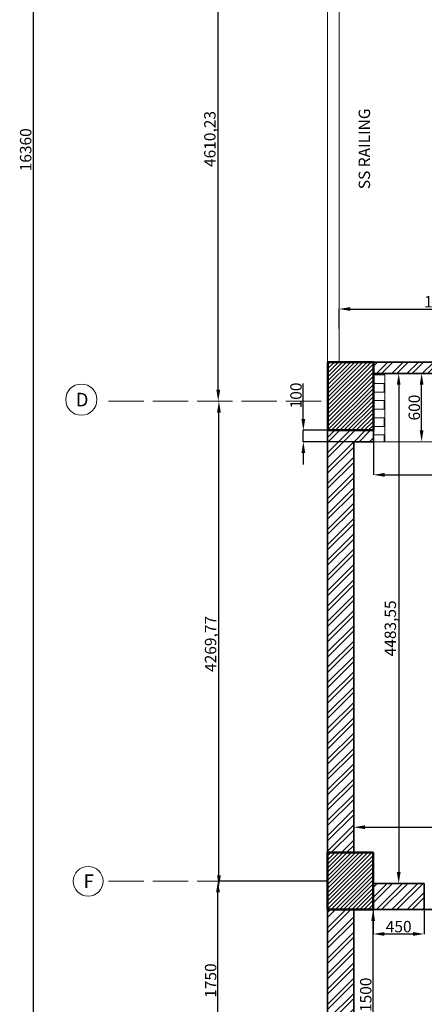
# Model space of a CAD drawing. Units: millimetres. Extents: x -3326 to 29338, y -16792 to 6002.
# Tile 2 of 21: x -3326 to 233, y -12098 to -3440. Entities that reach past the tile are written whole.
import ezdxf

# ---------------------------------------------------------------- set-up
doc = ezdxf.new("R2010")
doc.units = ezdxf.units.MM
doc.header["$PDMODE"] = 35
doc.header["$PDSIZE"] = 5
doc.linetypes.add('ACAD_ISO04W100', pattern=[30, 24, -3, 0, -3])
for name, color, linetype, lineweight in [('A-ANNO-DIMS', 2, 'Continuous', 13), ('A-COLS', 1, 'Continuous', 50), ('A-COLS-PATT', 251, 'Continuous', 13), ('A-FLOR-CASE', 30, 'Continuous', 18), ('A-FLOR-CASE-PATT', 252, 'Continuous', 13), ('A-FLOR-RAIL', 8, 'Continuous', 20), ('A-GRID', 8, 'ACAD_ISO04W100', 13), ('A-GRID-IDEN', 7, 'Continuous', 18), ('A-WALL', 7, 'Continuous', 35), ('A-WALL-PATT', 252, 'Continuous', 13), ('txt', 7, 'Continuous', 18)]:
    doc.layers.add(name, color=color, linetype=linetype, lineweight=lineweight)
doc.styles.get("Standard").update_dxf_attribs({"font": 'arial.ttf'})
doc.dimstyles.new('ISO-25', dxfattribs={"dimtxt": 100, "dimasz": 100, "dimexe": 1.25, "dimexo": 0.625, "dimtad": 1, "dimtxsty": 'Standard', "dimcen": 2.5, "dimadec": 0, "dimazin": 0, "dimtfac": 1, "dimtmove": 0, "dimatfit": 3, "dimfxl": 1, "dimarcsym": 0})

# ---------------------------------------------------------------- blocks, each defined once
blk = doc.blocks.new('*D73')
at = {"layer": 'A-ANNO-DIMS', "color": 0, "lineweight": -2, "transparency": 16777216}
for p, q in [((-217.7, -11264.6), (-217.7, -11480.2)), ((232.3, -11264.6), (232.3, -11480.2)), ((-117.7, -11479), (132.3, -11479))]:
    blk.add_line(p, q, dxfattribs=at)
at = {"layer": 'A-ANNO-DIMS', "color": 0, "transparency": 16777216}
for points in [[(-117.7, -11462.3), (-117.7, -11495.7), (-217.7, -11479)], [(132.3, -11462.3), (132.3, -11495.7), (232.3, -11479)]]:
    blk.add_solid(points, dxfattribs=at)
at = {"layer": 'Defpoints', "color": 0, "transparency": 16777216}
for p in [(-217.7, -11264), (232.3, -11264), (232.3, -11479)]:
    blk.add_point(p, dxfattribs=at)
at = {"layer": 'A-ANNO-DIMS', "color": 0, "transparency": 16777216, "insert": (7.3, -11427.3), "char_height": 100, "attachment_point": 5}
blk.add_mtext('450', dxfattribs=at)
blk = doc.blocks.new('*D74')
at = {"layer": 'A-ANNO-DIMS', "color": 0, "lineweight": -2, "transparency": 16777216}
for p, q in [((-387.1, -11264), (-216.4, -11264)), ((-217.7, -12664), (-217.7, -11364)), ((-387.1, -12764), (-216.4, -12764))]:
    blk.add_line(p, q, dxfattribs=at)
at = {"layer": 'A-ANNO-DIMS', "color": 0, "transparency": 16777216}
for points in [[(-234.4, -11364), (-201, -11364), (-217.7, -11264)], [(-234.4, -12664), (-201, -12664), (-217.7, -12764)]]:
    blk.add_solid(points, dxfattribs=at)
at = {"layer": 'Defpoints', "color": 0, "transparency": 16777216}
for p in [(-387.7, -11264), (-217.7, -11264), (-387.7, -12764)]:
    blk.add_point(p, dxfattribs=at)
at = {"layer": 'A-ANNO-DIMS', "color": 0, "transparency": 16777216, "insert": (-269.4, -12014), "char_height": 100, "attachment_point": 5, "rotation": 90}
blk.add_mtext('1500', dxfattribs=at)
blk = doc.blocks.new('*D76')
at = {"layer": 'A-ANNO-DIMS', "color": 0, "lineweight": -2, "transparency": 16777216}
for p, q in [((-387.7, -10539.9), (-387.7, -10539.2)), ((-287.7, -10540.5), (3512.3, -10540.5)), ((3612.3, -10539.9), (3612.3, -10539.2))]:
    blk.add_line(p, q, dxfattribs=at)
at = {"layer": 'A-ANNO-DIMS', "color": 0, "transparency": 16777216}
for points in [[(-287.7, -10523.8), (-287.7, -10557.2), (-387.7, -10540.5)], [(3512.3, -10523.8), (3512.3, -10557.2), (3612.3, -10540.5)]]:
    blk.add_solid(points, dxfattribs=at)
at = {"layer": 'Defpoints', "color": 0, "transparency": 16777216}
for p in [(-387.7, -10540.5), (3612.3, -10540.5), (3612.3, -10540.5)]:
    blk.add_point(p, dxfattribs=at)
at = {"layer": 'A-ANNO-DIMS', "color": 0, "transparency": 16777216, "insert": (1612.3, -10488.8), "char_height": 100, "attachment_point": 5}
blk.add_mtext('4000', dxfattribs=at)
blk = doc.blocks.new('*D77')
at = {"layer": 'A-ANNO-DIMS', "color": 0, "lineweight": -2, "transparency": 16777216}
for p, q in [((-114.9, -6550.4), (8.6, -6550.4)), ((7.3, -6650.4), (7.3, -10934)), ((6.7, -11034), (6.1, -11034))]:
    blk.add_line(p, q, dxfattribs=at)
at = {"layer": 'A-ANNO-DIMS', "color": 0, "transparency": 16777216}
for points in [[(-9.4, -6650.4), (24, -6650.4), (7.3, -6550.4)], [(-9.4, -10934), (24, -10934), (7.3, -11034)]]:
    blk.add_solid(points, dxfattribs=at)
at = {"layer": 'Defpoints', "color": 0, "transparency": 16777216}
for p in [(-115.5, -6550.4), (7.3, -11034), (7.3, -11034)]:
    blk.add_point(p, dxfattribs=at)
at = {"layer": 'A-ANNO-DIMS', "color": 0, "transparency": 16777216, "insert": (-53.4, -8792.2), "char_height": 100, "attachment_point": 5, "rotation": 90}
blk.add_mtext('4483,55', dxfattribs=at)
blk = doc.blocks.new('*D78')
at = {"layer": 'A-ANNO-DIMS', "color": 0, "lineweight": -2, "transparency": 16777216}
for p, q in [((-215.5, -7151), (-215.5, -7443)), ((2559.5, -7151), (2559.5, -7443)), ((-115.5, -7441.8), (2459.5, -7441.8))]:
    blk.add_line(p, q, dxfattribs=at)
at = {"layer": 'A-ANNO-DIMS', "color": 0, "transparency": 16777216}
for points in [[(-115.5, -7425.1), (-115.5, -7458.5), (-215.5, -7441.8)], [(2459.5, -7425.1), (2459.5, -7458.5), (2559.5, -7441.8)]]:
    blk.add_solid(points, dxfattribs=at)
at = {"layer": 'Defpoints', "color": 0, "transparency": 16777216}
for p in [(-215.5, -7150.4), (2559.5, -7150.4), (2559.5, -7441.8)]:
    blk.add_point(p, dxfattribs=at)
at = {"layer": 'A-ANNO-DIMS', "color": 0, "transparency": 16777216, "insert": (1172, -7390.1), "char_height": 100, "attachment_point": 5}
blk.add_mtext('2775', dxfattribs=at)
blk = doc.blocks.new('*D79')
at = {"layer": 'A-ANNO-DIMS', "color": 0, "lineweight": -2, "transparency": 16777216}
for p, q in [((-831.6, -6950.4), (-831.6, -6638)), ((-216.1, -7050.4), (-832.9, -7050.4)), ((-831.6, -7150.4), (-831.6, -7050.4)), ((-216.1, -7150.4), (-832.9, -7150.4)), ((-831.6, -7250.4), (-831.6, -7350.4))]:
    blk.add_line(p, q, dxfattribs=at)
at = {"layer": 'A-ANNO-DIMS', "color": 0, "transparency": 16777216}
for points in [[(-848.3, -6950.4), (-814.9, -6950.4), (-831.6, -7050.4)], [(-848.3, -7250.4), (-814.9, -7250.4), (-831.6, -7150.4)]]:
    blk.add_solid(points, dxfattribs=at)
at = {"layer": 'Defpoints', "color": 0, "transparency": 16777216}
for p in [(-831.6, -7050.4), (-215.5, -7050.4), (-215.5, -7150.4)]:
    blk.add_point(p, dxfattribs=at)
at = {"layer": 'A-ANNO-DIMS', "color": 0, "transparency": 16777216, "insert": (-883.3, -6744.2), "char_height": 100, "attachment_point": 5, "rotation": 90}
blk.add_mtext('100', dxfattribs=at)
blk = doc.blocks.new('*D80')
at = {"layer": 'A-ANNO-DIMS', "color": 0, "lineweight": -2, "transparency": 16777216}
for p, q in [((209.6, -6550.4), (210.2, -6550.4)), ((208.9, -7050.4), (208.9, -6650.4)), ((209.6, -7150.4), (210.2, -7150.4))]:
    blk.add_line(p, q, dxfattribs=at)
at = {"layer": 'A-ANNO-DIMS', "color": 0, "transparency": 16777216}
for points in [[(192.3, -6650.4), (225.6, -6650.4), (208.9, -6550.4)], [(192.3, -7050.4), (225.6, -7050.4), (208.9, -7150.4)]]:
    blk.add_solid(points, dxfattribs=at)
at = {"layer": 'Defpoints', "color": 0, "transparency": 16777216}
for p in [(208.9, -6550.4), (208.9, -6550.4), (208.9, -7150.4)]:
    blk.add_point(p, dxfattribs=at)
at = {"layer": 'A-ANNO-DIMS', "color": 0, "transparency": 16777216, "insert": (157.2, -6850.4), "char_height": 100, "attachment_point": 5, "rotation": 90}
blk.add_mtext('600', dxfattribs=at)
blk = doc.blocks.new('*D87')
at = {"layer": 'A-ANNO-DIMS', "color": 0, "lineweight": -2, "transparency": 16777216}
for p, q in [((-517.7, -6155.6), (-517.7, -5982.7)), ((-417.7, -5984), (1182.3, -5984)), ((1282.3, -6155.6), (1282.3, -5982.7))]:
    blk.add_line(p, q, dxfattribs=at)
at = {"layer": 'A-ANNO-DIMS', "color": 0, "transparency": 16777216}
for points in [[(-417.7, -5967.3), (-417.7, -6000.6), (-517.7, -5984)], [(1182.3, -5967.3), (1182.3, -6000.6), (1282.3, -5984)]]:
    blk.add_solid(points, dxfattribs=at)
at = {"layer": 'Defpoints', "color": 0, "transparency": 16777216}
for p in [(1282.3, -5984), (-517.7, -6156.3), (1282.3, -6156.3)]:
    blk.add_point(p, dxfattribs=at)
at = {"layer": 'A-ANNO-DIMS', "color": 0, "transparency": 16777216, "insert": (382.3, -5932.3), "char_height": 100, "attachment_point": 5}
blk.add_mtext('1800', dxfattribs=at)
blk = doc.blocks.new('*D162')
at = {"layer": 'A-ANNO-DIMS', "color": 0, "lineweight": -2, "transparency": 16777216}
for p, q in [((-618.3, -11014), (-1583.4, -11014)), ((-1582.2, -12664), (-1582.2, -11114)), ((-618.3, -12764), (-1583.4, -12764))]:
    blk.add_line(p, q, dxfattribs=at)
at = {"layer": 'A-ANNO-DIMS', "color": 0, "transparency": 16777216}
for points in [[(-1598.8, -11114), (-1565.5, -11114), (-1582.2, -11014)], [(-1598.8, -12664), (-1565.5, -12664), (-1582.2, -12764)]]:
    blk.add_solid(points, dxfattribs=at)
at = {"layer": 'Defpoints', "color": 0, "transparency": 16777216}
for p in [(-1582.2, -11014), (-617.7, -11014), (-617.7, -12764)]:
    blk.add_point(p, dxfattribs=at)
at = {"layer": 'A-ANNO-DIMS', "color": 0, "transparency": 16777216, "insert": (-1633.8, -11889), "char_height": 100, "attachment_point": 5, "rotation": 90}
blk.add_mtext('1750', dxfattribs=at)
blk = doc.blocks.new('*D163')
at = {"layer": 'A-ANNO-DIMS', "color": 0, "lineweight": -2, "transparency": 16777216}
for p, q in [((-1574.5, -6794.2), (-1575.1, -6794.2)), ((-1573.8, -10964), (-1573.8, -6894.2)), ((-1574.5, -11064), (-1575.1, -11064))]:
    blk.add_line(p, q, dxfattribs=at)
at = {"layer": 'A-ANNO-DIMS', "color": 0, "transparency": 16777216}
for points in [[(-1590.5, -6894.2), (-1557.2, -6894.2), (-1573.8, -6794.2)], [(-1590.5, -10964), (-1557.2, -10964), (-1573.8, -11064)]]:
    blk.add_solid(points, dxfattribs=at)
at = {"layer": 'Defpoints', "color": 0, "transparency": 16777216}
for p in [(-1573.8, -6794.2), (-1573.8, -6794.2), (-1573.8, -11064)]:
    blk.add_point(p, dxfattribs=at)
at = {"layer": 'A-ANNO-DIMS', "color": 0, "transparency": 16777216, "insert": (-1634.6, -8929.1), "char_height": 100, "attachment_point": 5, "rotation": 90}
blk.add_mtext('4269,77', dxfattribs=at)
blk = doc.blocks.new('*D164')
at = {"layer": 'A-ANNO-DIMS', "color": 0, "lineweight": -2, "transparency": 16777216}
for p, q in [((-1580.6, -2184), (-1581.2, -2184)), ((-1580, -6694.2), (-1580, -2284)), ((-1581.5, -6794.2), (-1578.7, -6794.2))]:
    blk.add_line(p, q, dxfattribs=at)
at = {"layer": 'A-ANNO-DIMS', "color": 0, "transparency": 16777216}
for points in [[(-1596.7, -2284), (-1563.3, -2284), (-1580, -2184)], [(-1596.7, -6694.2), (-1563.3, -6694.2), (-1580, -6794.2)]]:
    blk.add_solid(points, dxfattribs=at)
at = {"layer": 'Defpoints', "color": 0, "transparency": 16777216}
for p in [(-1580, -2184), (-1580, -2184), (-1582.2, -6794.2)]:
    blk.add_point(p, dxfattribs=at)
at = {"layer": 'A-ANNO-DIMS', "color": 0, "transparency": 16777216, "insert": (-1640.7, -4489.1), "char_height": 100, "attachment_point": 5, "rotation": 90}
blk.add_mtext('4610,23', dxfattribs=at)
blk = doc.blocks.new('*D167')
at = {"layer": 'A-ANNO-DIMS', "color": 0, "lineweight": -2, "transparency": 16777216}
for p, q in [((-618.3, 3596), (-3210.3, 3596)), ((-3209, 3496), (-3209, -12664)), ((-618.3, -12764), (-3210.3, -12764))]:
    blk.add_line(p, q, dxfattribs=at)
at = {"layer": 'A-ANNO-DIMS', "color": 0, "transparency": 16777216}
for points in [[(-3225.7, 3496), (-3192.4, 3496), (-3209, 3596)], [(-3225.7, -12664), (-3192.4, -12664), (-3209, -12764)]]:
    blk.add_solid(points, dxfattribs=at)
at = {"layer": 'Defpoints', "color": 0, "transparency": 16777216}
for p in [(-617.7, 3596), (-3209, -12764), (-617.7, -12764)]:
    blk.add_point(p, dxfattribs=at)
at = {"layer": 'A-ANNO-DIMS', "color": 0, "transparency": 16777216, "insert": (-3260.8, -4584), "char_height": 100, "attachment_point": 5, "rotation": 90}
blk.add_mtext('16360', dxfattribs=at)

msp = doc.modelspace()

# ---------------------------------------------------------------- hatches: boundary and pattern name
at = {"layer": 'A-COLS-PATT'}
h = msp.add_hatch(dxfattribs=at)
h.set_pattern_fill('ANSI31', color=256, scale=8)
h.set_pattern_definition([(45, (-42336.819, 156.603), (-17.960512, 17.960512), [])])
h.paths.add_polyline_path([(-615.519, -7050.401), (-215.519, -7050.401), (-215.519, -6450.401), (-615.519, -6450.401)])
h = msp.add_hatch(dxfattribs=at)
h.set_pattern_fill('ANSI31', color=256, scale=8)
h.set_pattern_definition([(45, (-45233.41, -5550.314), (-17.960512, 17.960512), [])])
h.paths.add_polyline_path([(-617.699, -10763.952), (-617.699, -11263.952), (-217.699, -11263.952), (-217.699, -10763.952)])
at = {"layer": 'A-FLOR-CASE-PATT'}
h = msp.add_hatch(dxfattribs=at)
h.set_pattern_fill('BRSTONE', color=256, scale=9)
h.set_pattern_definition([(0, (-10476.645, 1e-12), (0, 75.438), []), (90, (-10270.9, 1e-12), (-114.3, 75.438), [75.438, -75.438]), (90, (-10293.77, 1e-12), (-114.3, 75.438), [75.438, -75.438]), (0, (-10270.905, 12.57), (114.3, 75.438), [-205.74, 22.86]), (0, (-10270.905, 25.146), (114.3, 75.438), [-205.74, 22.86]), (0, (-10270.905, 37.72), (114.3, 75.438), [-205.74, 22.86]), (0, (-10270.905, 50.29), (114.3, 75.438), [-205.74, 22.86]), (0, (-10270.905, 62.865), (114.3, 75.438), [-205.74, 22.86])])
h.paths.add_polyline_path([(-115.519, -6550.401), (-215.519, -6550.401), (-215.519, -7050.401), (-215.519, -7150.401), (-115.519, -7150.401)])
h.paths.add_polyline_path([(792.814, -6550.401), (692.814, -6550.401), (692.814, -7150.401), (792.814, -7150.401)])
h.paths.add_polyline_path([(1651.147, -6550.401), (1551.147, -6550.401), (1551.147, -7150.401), (1651.147, -7150.401)])
h.paths.add_polyline_path([(2559.481, -6550.401), (2459.481, -6550.401), (2459.481, -7150.401), (2559.481, -7150.401)])
at = {"layer": 'A-WALL-PATT'}
h = msp.add_hatch(dxfattribs=at)
h.set_pattern_fill('ANSI32', color=256, scale=10)
h.set_pattern_definition([(45, (-10476.65, 1e-12), (-67.35192, 67.35192), []), (45, (-10431.74, 1e-12), (-67.35192, 67.35192), [])])
h.paths.add_polyline_path([(7302.301, -11263.952), (7902.301, -11263.952), (7902.301, -11033.952), (7302.301, -11033.952), (7302.301, -8110.991), (7202.301, -8110.991), (7202.301, -11033.952), (6672.301, -11033.952), (6672.301, -11263.952), (7072.301, -11263.952), (7072.301, -12763.952), (7302.301, -12763.952)])
h.paths.add_polyline_path([(9152.301, -11033.952), (8802.301, -11033.952), (8802.301, -11044.19), (8802.545, -11044.19), (8802.545, -11124.19), (8802.301, -11263.952), (9152.301, -11263.952)])
h.paths.add_polyline_path([(3712.301, -8110.991), (3612.301, -8110.991), (3612.301, -11033.952), (3282.301, -11033.952), (3282.301, -11263.952), (3612.301, -11263.952), (3612.301, -12763.952), (3842.301, -12763.952), (3842.301, -11263.952), (4092.301, -11263.952), (4092.301, -11033.952), (3842.301, -11033.952), (3712.301, -11033.952)])
h.paths.add_polyline_path([(5172.301, -11033.952), (4692.301, -11033.952), (4692.301, -11263.952), (5172.301, -11263.952)])
h.paths.add_polyline_path([(6072.301, -11033.952), (5572.301, -11033.952), (5572.301, -11263.952), (6072.301, -11263.952)])
h.paths.add_polyline_path([(6072.301, -11263.952), (5972.301, -11263.952), (5972.301, -11663.952), (6072.301, -11663.952)])
h.paths.add_polyline_path([(4792.301, -11263.952), (4692.301, -11263.952), (4692.301, -11663.952), (4792.301, -11663.952)])
h.paths.add_polyline_path([(6402.301, -8110.991), (6272.301, -8110.991), (5572.301, -8110.991), (5572.301, -7200.401), (5342.301, -7200.401), (5342.301, -8110.991), (4642.301, -8110.991), (4512.301, -8110.991), (4512.301, -8210.991), (4642.301, -8210.991), (5342.301, -8210.991), (5342.301, -10513.952), (5572.301, -10513.952), (5572.301, -8210.991), (6272.301, -8210.991), (6402.301, -8210.991)])
h.paths.add_polyline_path([(232.301, -11033.952), (-217.699, -11033.952), (-217.699, -11263.952), (232.301, -11263.952)])
h.paths.add_polyline_path([(1482.301, -11033.952), (1132.301, -11033.952), (1132.301, -11044.8), (1132.987, -11044.8), (1132.987, -11124.8), (1132.301, -11263.952), (1482.301, -11263.952)])
h.paths.add_polyline_path([(-387.699, -11263.952), (-617.699, -11263.952), (-617.699, -12763.952), (-438.882, -12763.952), (-387.699, -12763.952)])
h.paths.add_polyline_path([(-387.699, -7150.401), (-215.519, -7150.401), (-215.519, -7050.401), (-617.699, -7050.401), (-617.699, -10763.952), (-387.699, -10763.952)])
h.paths.add_polyline_path([(1512.301, -5983.952), (1282.301, -5983.952), (1282.301, -6450.401), (-215.519, -6450.401), (-215.519, -6550.401), (4073.51, -6550.401), (4073.51, -6450.401), (1512.301, -6450.401)])
h.paths.add_polyline_path([(5773.51, -6450.401), (5573.51, -6450.401), (5573.51, -6550.401), (5773.51, -6550.401)])
h.paths.add_polyline_path([(5173.51, -6450.401), (4973.51, -6450.401), (4973.51, -6550.401), (5173.51, -6550.401)])
h.paths.add_polyline_path([(10982.301, -6450.401), (6673.51, -6450.401), (6673.51, -6550.401), (10982.301, -6550.401)])

# ---------------------------------------------------------------- linework, layer by layer
at = {"layer": 'A-COLS'}
for points in [[(-615.519, -6450.401), (-215.519, -6450.401), (-215.519, -7050.401), (-615.519, -7050.401)], [(-617.699, -10763.952), (-217.699, -10763.952), (-217.699, -11263.952), (-617.699, -11263.952)]]:
    msp.add_lwpolyline(points, close=True, dxfattribs=at)
at = {"layer": 'A-FLOR-CASE'}
for p, q in [((-115.519, -6550.401), (-115.519, -7150.401)), ((-215.519, -7150.401), (-115.519, -7150.401)), ((-115.519, -7150.401), (2459.481, -7150.401))]:
    msp.add_line(p, q, dxfattribs=at)
at = {"layer": 'A-FLOR-RAIL'}
for p, q in [((-617.699, -2483.952), (-617.699, -6450.401)), ((-517.699, -2483.952), (-517.699, -6450.401))]:
    msp.add_line(p, q, dxfattribs=at)
at = {"layer": 'A-GRID', "ltscale": 13}
for p, q in [((-2546.632, -6794.183), (-617.699, -6794.183)), ((-2546.632, -11013.952), (-617.699, -11013.952))]:
    msp.add_line(p, q, dxfattribs=at)
at = {"layer": 'A-GRID-IDEN'}
for centre, radius in [((-2784.067, -6780.801), 137.096), ((-2723.912, -11015.818), 131.174)]:
    msp.add_circle(centre, radius, dxfattribs=at)
at = {"layer": 'A-WALL'}
for p, q in [((-617.699, -6450.401), (-617.699, -12763.952)), ((1282.301, -6450.401), (-387.699, -6450.401)), ((4073.51, -6550.401), (-215.519, -6550.401)), ((-215.519, -7050.401), (-215.519, -7150.401)), ((-387.699, -7150.401), (-387.699, -10763.952)), ((-215.519, -7150.401), (-387.699, -7150.401)), ((232.301, -11033.952), (-217.699, -11033.952)), ((232.301, -11033.952), (232.301, -11263.952)), ((-387.699, -11263.952), (-387.699, -12763.952)), ((3612.301, -11263.952), (-217.699, -11263.952))]:
    msp.add_line(p, q, dxfattribs=at)

# ---------------------------------------------------------------- texts
at = {"layer": 'A-GRID-IDEN', "char_height": 120, "attachment_point": 1}
for s, insert in [('D', (-2833.672, -6720.801)), ('F', (-2764.39, -10955.818))]:
    msp.add_mtext_dynamic_manual_height_columns(s, width=319.52755, gutter_width=12.5, heights=[0], dxfattribs=dict(at, insert=insert))
at = {"layer": 'txt', "insert": (-344.762, -4930.339), "char_height": 100, "attachment_point": 1, "rotation": 90}
msp.add_mtext_dynamic_manual_height_columns('SS RAILING', width=1168.90663, gutter_width=12.5, heights=[0], dxfattribs=at)

# ---------------------------------------------------------------- dimensions: what is measured, and where the dimension line sits
at = {"layer": 'A-ANNO-DIMS'}
for base, p1, p2, picture, middle in [((-3209.046, -12763.952), (-617.699, 3596.048), (-617.699, -12763.952), '*D167', (-3260.762, -4583.952)), ((-1579.986, -2183.952), (-1582.166, -6794.183), (-1579.986, -2183.952), '*D164', (-1640.706, -4489.067)), ((7.301, -11033.952), (-115.519, -6550.401), (7.301, -11033.952), '*D77', (-53.42, -8792.177)), ((208.927, -6550.401), (208.927, -7150.401), (208.927, -6550.401), '*D80', (157.245, -6850.401)), ((-831.607, -7050.401), (-215.519, -7150.401), (-215.519, -7050.401), '*D79', (-883.289, -6744.183)), ((-1573.832, -6794.183), (-1573.832, -11063.952), (-1573.832, -6794.183), '*D163', (-1634.553, -8929.067)), ((-1582.166, -11013.952), (-617.699, -12763.952), (-617.699, -11013.952), '*D162', (-1633.848, -11888.952)), ((-217.699, -11263.952), (-387.699, -12763.952), (-387.699, -11263.952), '*D74', (-269.382, -12013.952))]:
    dim = msp.add_linear_dim(base=base, p1=p1, p2=p2, angle=90, dimstyle='ISO-25', override={"dimclrd": 0, "dimclre": 0, "dimclrt": 0}, dxfattribs=at)
    dim.commit()
    dim.dimension.update_dxf_attribs({"geometry": picture, "text_midpoint": middle})
for base, p1, p2, picture, middle in [((1282.301, -5983.952), (-517.699, -6156.262), (1282.301, -6156.262), '*D87', (382.301, -5932.27)), ((2559.481, -7441.784), (-215.519, -7150.401), (2559.481, -7150.401), '*D78', (1171.981, -7390.102)), ((3612.301, -10540.499), (-387.699, -10540.499), (3612.301, -10540.499), '*D76', (1612.301, -10488.817)), ((232.301, -11478.994), (-217.699, -11263.952), (232.301, -11263.952), '*D73', (7.301, -11427.312))]:
    dim = msp.add_linear_dim(base=base, p1=p1, p2=p2, dimstyle='ISO-25', override={"dimclrd": 0, "dimclre": 0, "dimclrt": 0}, dxfattribs=at)
    dim.commit()
    dim.dimension.update_dxf_attribs({"geometry": picture, "text_midpoint": middle})

doc.saveas('drawing.dxf')
